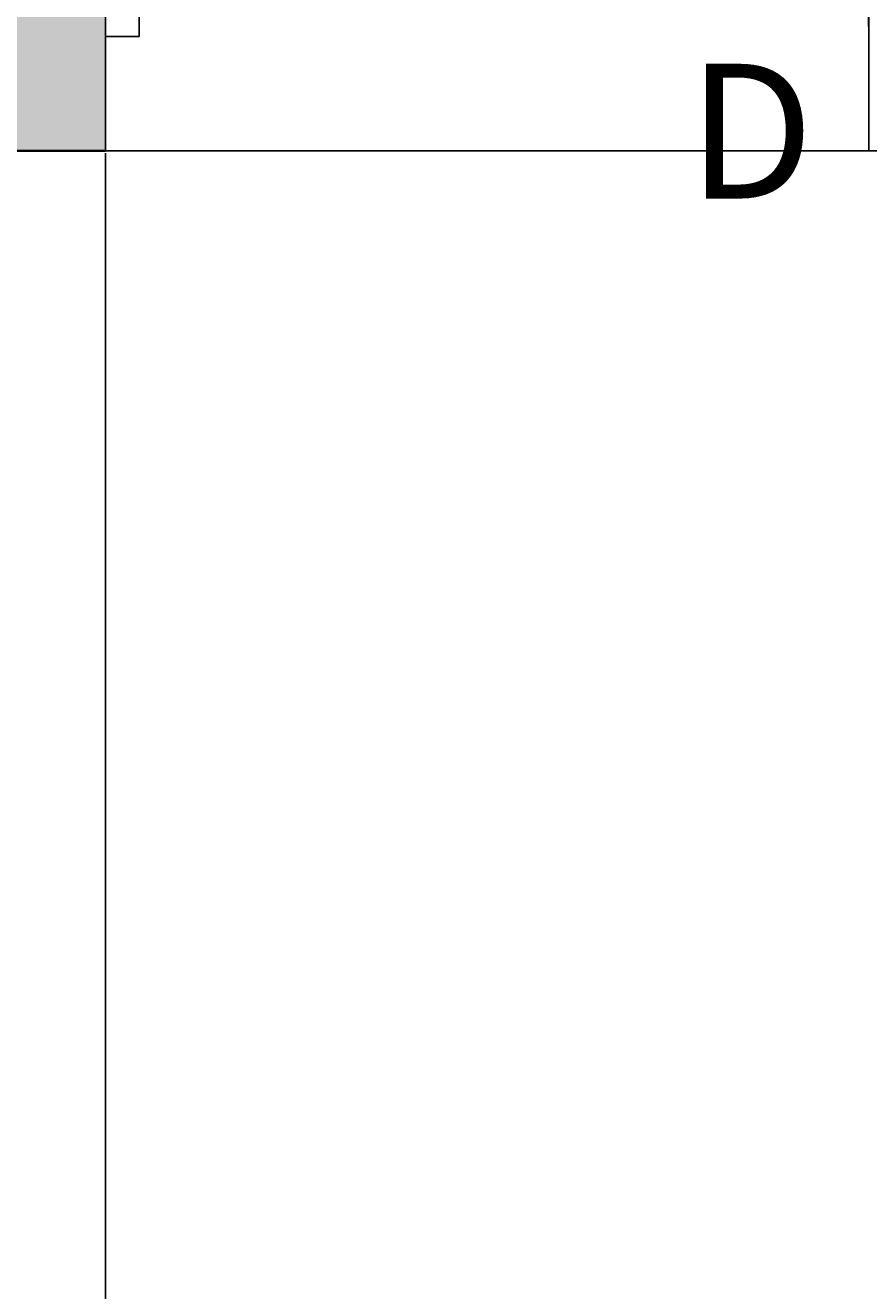
# Model space of a CAD drawing. Units: inches. Extents: x 1998 to 2588, y 1139 to 1977.
# Tile 41 of 134: x 2293 to 2316, y 1557 to 1592. Entities that reach past the tile are written whole.
import ezdxf

# ---------------------------------------------------------------- set-up
doc = ezdxf.new("R2010")
doc.units = ezdxf.units.IN
for name, color, linetype, lineweight in [('A-ANNO-DIMS', 2, 'Continuous', 18), ('A-DOOR-IDEN', 7, 'Continuous', 18), ('A-WALL-PATT', 252, 'Continuous', 13), ('DOOR', 52, 'Continuous', 25), ('WALL', 200, 'Continuous', 35)]:
    doc.layers.add(name, color=color, linetype=linetype, lineweight=lineweight)
doc.styles.get("Standard").update_dxf_attribs({"font": 'arial.ttf'})
doc.dimstyles.get("Standard").update_dxf_attribs({"dimtxt": 0.18, "dimasz": 0.18, "dimexe": 0.18, "dimexo": 0.0625, "dimgap": 0.09, "dimtad": 0, "dimtih": 1, "dimtoh": 1, "dimdec": 4, "dimzin": 0, "dimdsep": 46, "dimtxsty": 'Standard', "dimcen": 0.09, "dimadec": 0, "dimazin": 0, "dimtfac": 1, "dimtdec": 4, "dimtofl": 0, "dimtmove": 0, "dimatfit": 3, "dimfxl": 1, "dimtolj": 1, "dimtzin": 0, "dimarcsym": 0})

# ---------------------------------------------------------------- blocks, each defined once
blk = doc.blocks.new('*U2')
for p, q in [((0, 0), (0, -6)), ((40, 0), (40, -6))]:
    blk.add_line(p, q)
blk.add_lwpolyline([(0, 0), (0, 40), (1.75, 40), (1.75, 0)], close=True)
blk.add_arc((0, 0), 40, 0, 90)
blk = doc.blocks.new('*D34')
at = {"layer": 'A-ANNO-DIMS', "color": 0, "lineweight": -2, "transparency": 16777216}
for p, q in [((2407.91, 1594.732), (1997.843, 1594.732)), ((1998.023, 1594.552), (1998.023, 1558.913)), ((1998.023, 1522.912), (1998.023, 1558.552)), ((2407.91, 1522.732), (1997.843, 1522.732))]:
    blk.add_line(p, q, dxfattribs=at)
at = {"layer": 'A-ANNO-DIMS', "color": 0, "transparency": 16777216}
for points in [[(1997.993, 1594.552), (1998.053, 1594.552), (1998.023, 1594.732)], [(1997.993, 1522.912), (1998.053, 1522.912), (1998.023, 1522.732)]]:
    blk.add_solid(points, dxfattribs=at)
at = {"layer": 'Defpoints', "color": 0, "transparency": 16777216}
for p in [(1998.023, 1594.732), (2407.973, 1594.732), (2407.973, 1522.732)]:
    blk.add_point(p, dxfattribs=at)
at = {"layer": 'A-ANNO-DIMS', "color": 0, "transparency": 16777216, "insert": (1998.023, 1558.732), "char_height": 0.18, "attachment_point": 5}
blk.add_mtext('\\A1;72', dxfattribs=at)
blk = doc.blocks.new('*D42')
at = {"layer": 'A-ANNO-DIMS', "color": 0, "lineweight": -2, "transparency": 16777216}
for p, q in [((2287.535, 1588.732), (2588.309, 1588.732)), ((2588.129, 1588.552), (2588.129, 1555.914)), ((2588.129, 1522.912), (2588.129, 1555.55)), ((2287.535, 1522.732), (2588.309, 1522.732))]:
    blk.add_line(p, q, dxfattribs=at)
at = {"layer": 'A-ANNO-DIMS', "color": 0, "transparency": 16777216}
for points in [[(2588.099, 1588.552), (2588.159, 1588.552), (2588.129, 1588.732)], [(2588.099, 1522.912), (2588.159, 1522.912), (2588.129, 1522.732)]]:
    blk.add_solid(points, dxfattribs=at)
at = {"layer": 'Defpoints', "color": 0, "transparency": 16777216}
for p in [(2287.473, 1588.732), (2588.129, 1588.732), (2287.473, 1522.732)]:
    blk.add_point(p, dxfattribs=at)
at = {"layer": 'A-ANNO-DIMS', "color": 0, "transparency": 16777216, "insert": (2588.129, 1555.732), "char_height": 0.18, "attachment_point": 5}
blk.add_mtext('\\A1;66', dxfattribs=at)
blk = doc.blocks.new('*D44')
at = {"layer": 'A-ANNO-DIMS', "color": 0, "lineweight": -2, "transparency": 16777216}
for p, q in [((2295.414, 1588.67), (2295.414, 1138.602)), ((2337.287, 1588.67), (2337.287, 1138.602)), ((2295.594, 1138.782), (2315.953, 1138.782)), ((2337.107, 1138.782), (2316.748, 1138.782))]:
    blk.add_line(p, q, dxfattribs=at)
at = {"layer": 'A-ANNO-DIMS', "color": 0, "transparency": 16777216}
for points in [[(2295.594, 1138.812), (2295.594, 1138.752), (2295.414, 1138.782)], [(2337.107, 1138.812), (2337.107, 1138.752), (2337.287, 1138.782)]]:
    blk.add_solid(points, dxfattribs=at)
at = {"layer": 'Defpoints', "color": 0, "transparency": 16777216}
for p in [(2295.414, 1588.732), (2337.287, 1588.732), (2337.287, 1138.782)]:
    blk.add_point(p, dxfattribs=at)
at = {"layer": 'A-ANNO-DIMS', "color": 0, "transparency": 16777216, "insert": (2316.35, 1138.782), "char_height": 0.18, "attachment_point": 5}
blk.add_mtext('\\A1;41.87', dxfattribs=at)

msp = doc.modelspace()

# ---------------------------------------------------------------- hatches: boundary and pattern name
at = {"layer": 'A-WALL-PATT'}
h = msp.add_hatch(color=256, dxfattribs=at)
h.dxf.hatch_style = 1
h.paths.add_polyline_path([(2222.9729, 1888.7324), (2099.4125, 1888.7324), (2099.4125, 1879.7324), (2222.9729, 1879.7324)])
h.paths.add_polyline_path([(2096.9729, 1868.3278), (2087.9729, 1868.3278), (2087.9729, 1775.637), (2096.9729, 1775.637)])
h.paths.add_polyline_path([(2227.4729, 1868.3278), (2222.9729, 1868.3278), (2222.9729, 1774.3318), (2227.4729, 1774.3318)])
h.paths.add_polyline_path([(2188.3019, 1759.7324), (2138.6074, 1759.7324), (2099.4125, 1759.7324), (2099.4125, 1755.2324), (2176.9729, 1755.2324), (2188.3019, 1755.2324)])
h.paths.add_polyline_path([(2087.9729, 1759.7324), (2059.4729, 1759.7324), (2059.4729, 1702.7324), (2087.9729, 1702.7324), (2087.9729, 1707.2324), (2063.9729, 1707.2324), (2063.9729, 1755.2324), (2087.9729, 1755.2324)])
h.paths.add_polyline_path([(2096.9729, 1755.2324), (2087.9729, 1755.2324), (2087.9729, 1707.2324), (2096.9729, 1707.2324)])
h.paths.add_polyline_path([(2187.0461, 1707.2324), (2105.9729, 1707.2324), (2096.9729, 1707.2324), (2087.9729, 1707.2324), (2087.9729, 1702.7324), (2105.9729, 1702.7324), (2114.9729, 1702.7324), (2187.0461, 1702.7324)])
h.paths.add_polyline_path([(2181.4729, 1719.2028), (2176.9729, 1719.2028), (2176.9729, 1707.2324), (2181.4729, 1707.2324)])
h.paths.add_polyline_path([(2216.0332, 1588.7324), (2114.9729, 1588.7324), (2105.9729, 1588.7324), (2105.9729, 1584.2324), (2216.0332, 1584.2324)])
h.paths.add_polyline_path([(2077.691, 1588.7324), (2061.4729, 1588.7324), (2061.4729, 1584.2324), (2077.691, 1584.2324)])
h.paths.add_polyline_path([(2105.9729, 1588.7324), (2098.0956, 1588.7324), (2098.0956, 1584.2324), (2105.9729, 1584.2324)])
h.paths.add_polyline_path([(2114.9729, 1596.2642), (2110.1012, 1596.2642), (2105.9729, 1596.2642), (2105.9729, 1588.7324), (2114.9729, 1588.7324)])
h.paths.add_polyline_path([(2114.9729, 1584.2324), (2105.9729, 1584.2324), (2105.9729, 1580.249), (2110.1012, 1580.249), (2114.9729, 1580.249)])
h.paths.add_polyline_path([(2114.9729, 1547.7716), (2110.1012, 1547.7716, -0.0318759), (2105.9729, 1548.035), (2105.9729, 1470.2324), (2108.3775, 1470.2324), (2108.3775, 1465.7324), (2186.2943, 1465.7324), (2186.2943, 1470.2324), (2114.9729, 1470.2324)])
h.paths.add_polyline_path([(2227.4729, 1584.2324), (2222.9729, 1584.2324), (2222.9729, 1486.137), (2227.4729, 1486.137)])
h.paths.add_polyline_path([(2295.4138, 1593.2324), (2227.4729, 1593.2324), (2227.4729, 1588.7324), (2295.4138, 1588.7324), (2295.4138, 1591.8729)])
h.paths.add_polyline_path([(2345.9729, 1627.1165), (2341.4729, 1627.1165), (2341.4729, 1593.2324), (2337.2869, 1593.2324), (2337.2869, 1591.8729), (2337.2869, 1588.7324), (2345.9729, 1588.7324)])
h.paths.add_polyline_path([(2291.9729, 1588.7324), (2287.4729, 1588.7324), (2287.4729, 1522.7324), (2291.9729, 1522.7324)])
h.paths.add_polyline_path([(2291.9729, 1522.7324), (2287.4729, 1522.7324), (2227.4729, 1522.7324), (2227.4729, 1518.2324), (2291.9729, 1518.2324)])
h.paths.add_polyline_path([(2295.7347, 1519.5919), (2295.7347, 1522.7324), (2291.9729, 1522.7324), (2291.9729, 1518.2324), (2295.7347, 1518.2324)])
h.paths.add_polyline_path([(2345.9729, 1522.7324), (2337.6078, 1522.7324), (2337.6078, 1519.5919), (2337.6078, 1518.2324), (2341.4729, 1518.2324), (2341.4729, 1488.5616), (2345.9729, 1488.5616)])
h.paths.add_polyline_path([(2345.9729, 1468.1569), (2341.4729, 1468.1569), (2341.4729, 1374.2324), (2227.4729, 1374.2324), (2227.4729, 1369.7324), (2345.9729, 1369.7324)])
h.paths.add_polyline_path([(2345.9729, 1369.7324), (2341.4729, 1369.7324), (2341.4729, 1362.2324), (2345.9729, 1362.2324)])
h.paths.add_polyline_path([(2345.9729, 1317.7324), (2345.9729, 1322.2324), (2341.4729, 1322.2324), (2341.4729, 1285.137), (2345.9729, 1285.137)], flags=17)
h.paths.add_polyline_path([(2356.2096, 1322.2324), (2345.9729, 1322.2324), (2345.9729, 1317.7324), (2356.2096, 1317.7324), (2356.2096, 1319.3088)], flags=17)
h.paths.add_polyline_path([(2393.9729, 1322.2324), (2375.6999, 1322.2324), (2375.6999, 1319.3088, -0.0202458), (2375.636, 1317.7324), (2393.9729, 1317.7324)], flags=17)
h.paths.add_polyline_path([(2398.4729, 1322.2324), (2393.9729, 1322.2324), (2393.9729, 1317.7324), (2393.9729, 1237.7324), (2345.9729, 1237.7324), (2345.9729, 1264.7324), (2341.4729, 1264.7324), (2341.4729, 1228.7324), (2393.9729, 1228.7324), (2482.7412, 1228.7324), (2482.7412, 1237.7324), (2398.4729, 1237.7324), (2398.4729, 1297.1029)])
h.paths.add_polyline_path([(2398.4729, 1362.2324), (2393.9729, 1362.2324), (2393.9729, 1357.7324), (2398.4729, 1357.7324)])
h.paths.add_polyline_path([(2345.9729, 1329.7549), (2341.4729, 1329.7549), (2341.4729, 1322.2324), (2345.9729, 1322.2324)])

# ---------------------------------------------------------------- linework, layer by layer
at = {"layer": 'WALL'}
msp.add_line((2295.4138, 1588.7324), (2227.4729, 1588.7324), dxfattribs=at)

# ---------------------------------------------------------------- block references
at = {"layer": 'DOOR', "yscale": 0.5234138920659225, "zscale": 0.5234138920659225}
for p, xscale in [((2295.4138, 1591.8729), 0.5234138920659225), ((2337.2869, 1591.8729), -0.5234138920659225)]:
    msp.add_blockref('*U2', p, dxfattribs=dict(at, xscale=xscale))

# ---------------------------------------------------------------- texts
at = {"layer": 'A-DOOR-IDEN', "insert": (2311.38, 1591.121), "char_height": 3.6988, "attachment_point": 1}
msp.add_mtext_dynamic_manual_height_columns('D', width=110.572713, gutter_width=18.4938, heights=[0], dxfattribs=at)

# ---------------------------------------------------------------- dimensions: what is measured, and where the dimension line sits
at = {"layer": 'A-ANNO-DIMS'}
for base, p1, p2, picture, middle in [((1998.0229, 1594.7324), (2407.9729, 1522.7324), (2407.9729, 1594.7324), '*D34', (1998.0229, 1558.7324)), ((2588.1286, 1588.7324), (2287.4729, 1522.7324), (2287.4729, 1588.7324), '*D42', (2588.1286, 1555.7324))]:
    dim = msp.add_linear_dim(base=base, p1=p1, p2=p2, angle=90, dimstyle='Standard', override={"dimdec": 0, "dimlfac": 1, "dimrnd": 0, "dimzin": 0, "dimdsep": 46, "dimlunit": 2}, dxfattribs=at)
    dim.commit()
    dim.dimension.update_dxf_attribs({"geometry": picture, "text_midpoint": middle})
dim = msp.add_linear_dim(base=(2337.2869, 1138.7824), p1=(2295.4138, 1588.7324), p2=(2337.2869, 1588.7324), dimstyle='Standard', override={"dimdec": 2, "dimlfac": 1, "dimrnd": 0, "dimzin": 0, "dimdsep": 46, "dimlunit": 2}, dxfattribs=at)
dim.commit()
dim.dimension.update_dxf_attribs({"geometry": '*D44', "text_midpoint": (2316.3503, 1138.7824)})

doc.saveas('drawing.dxf')
